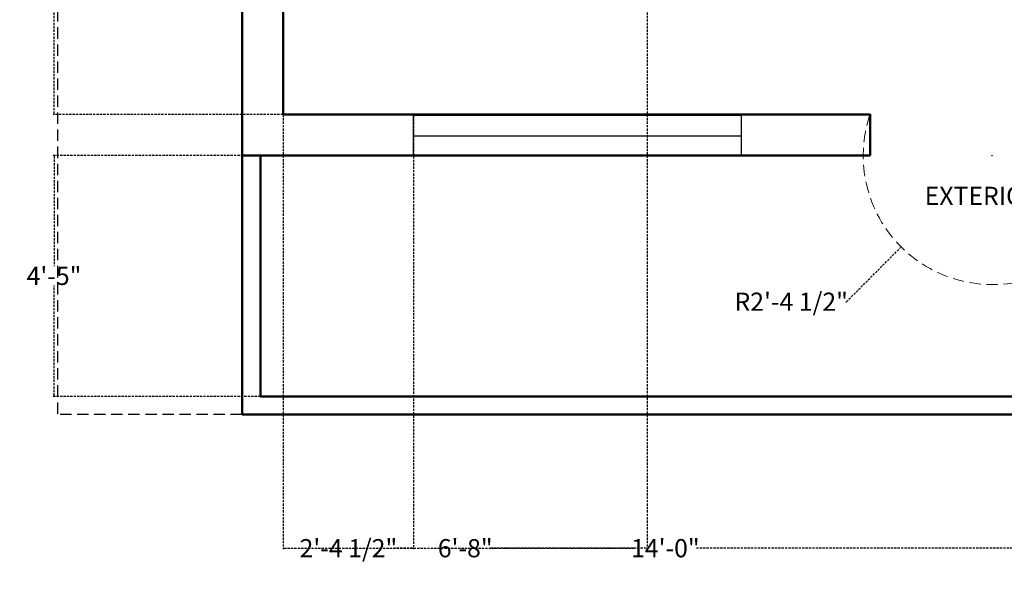
# Model space of a CAD drawing. Units: inches. Extents: x 513 to 1142, y 396 to 927.
# Tile 1 of 31: x 526 to 743, y 396 to 518. Entities that reach past the tile are written whole.
import ezdxf

# ---------------------------------------------------------------- set-up
doc = ezdxf.new("R2010")
doc.units = ezdxf.units.IN
doc.header["$MEASUREMENT"] = 0
doc.linetypes.add('DASHED', pattern=[0.75, 0.5, -0.25])
for name, color, linetype, lineweight in [('A-ANNO-DIMS', 2, 'DASHED', 18), ('A-DOOR-SWNG', 4, 'DASHED', 13), ('A-WALL', 7, 'Continuous', 50), ('windows', 172, 'Continuous', 25)]:
    doc.layers.add(name, color=color, linetype=linetype, lineweight=lineweight)
doc.styles.get("Standard").update_dxf_attribs({"font": 'arial.ttf'})
doc.dimstyles.get("Standard").update_dxf_attribs({"dimtxt": 4, "dimasz": 0.18, "dimexe": 0.18, "dimexo": 0.0625, "dimgap": 0.09, "dimtad": 0, "dimtih": 1, "dimtoh": 1, "dimdec": 0, "dimrnd": 6, "dimzin": 0, "dimdsep": 46, "dimlunit": 3, "dimtxsty": 'Standard', "dimcen": 0.09, "dimadec": 0, "dimazin": 0, "dimtfac": 1, "dimtdec": 0, "dimtofl": 0, "dimtmove": 0, "dimatfit": 3, "dimfxl": 1, "dimtolj": 1, "dimtzin": 0, "dimarcsym": 0})

# ---------------------------------------------------------------- blocks, each defined once
blk = doc.blocks.new('*D104')
at = {"layer": 'A-ANNO-DIMS', "color": 0, "lineweight": -2, "ltscale": 5, "transparency": 16777216}
for p, q in [((574.93, 879.16), (534.25, 879.16)), ((534.43, 878.98), (534.43, 657.29)), ((534.43, 431.34), (534.43, 653.02)), ((574.93, 431.16), (534.25, 431.16))]:
    blk.add_line(p, q, dxfattribs=at)
at = {"layer": 'A-ANNO-DIMS', "color": 0, "ltscale": 5, "transparency": 16777216}
for points in [[(534.4, 878.98), (534.46, 878.98), (534.43, 879.16)], [(534.4, 431.34), (534.46, 431.34), (534.43, 431.16)]]:
    blk.add_solid(points, dxfattribs=at)
at = {"layer": 'Defpoints', "color": 0, "ltscale": 5, "transparency": 16777216}
for p in [(575, 879.16), (534.43, 431.16), (575, 431.16)]:
    blk.add_point(p, dxfattribs=at)
at = {"layer": 'A-ANNO-DIMS', "color": 0, "ltscale": 5, "transparency": 16777216, "insert": (534.43, 655.16), "char_height": 4, "attachment_point": 5}
blk.add_mtext('\\A1;37\'-6"', dxfattribs=at)
blk = doc.blocks.new('WIN-72IN')
blk.add_line((0, 4.45), (72, 4.45))
blk.add_lwpolyline([(72, 9), (72, 0), (0, 0), (0, 9)], close=True)
blk = doc.blocks.new('*D125')
at = {"layer": 'A-ANNO-DIMS', "color": 0, "lineweight": -2, "transparency": 16777216}
for p, q in [((752.06, 497.26), (757.58, 497.26)), ((757.4, 497.08), (757.4, 481.42)), ((757.4, 461.44), (757.4, 477.1)), ((752.06, 461.26), (757.58, 461.26))]:
    blk.add_line(p, q, dxfattribs=at)
at = {"layer": 'A-ANNO-DIMS', "color": 0, "transparency": 16777216}
for points in [[(757.37, 497.08), (757.43, 497.08), (757.4, 497.26)], [(757.37, 461.44), (757.43, 461.44), (757.4, 461.26)]]:
    blk.add_solid(points, dxfattribs=at)
at = {"layer": 'Defpoints', "color": 0, "transparency": 16777216}
for p in [(752, 497.26), (757.4, 497.26), (752, 461.26)]:
    blk.add_point(p, dxfattribs=at)
at = {"layer": 'A-ANNO-DIMS', "color": 0, "transparency": 16777216, "insert": (757.4, 479.26), "char_height": 4, "attachment_point": 5}
blk.add_mtext('\\A1;EXTERIOR LEAF 3\'-0" TYP.', dxfattribs=at)
blk = doc.blocks.new('*D142')
at = {"layer": 'A-ANNO-DIMS', "color": 0, "lineweight": -2, "transparency": 16777216}
for p, q in [((583.93, 637.16), (533.42, 637.16)), ((533.6, 636.98), (533.6, 569.29)), ((533.6, 497.34), (533.6, 565.03)), ((583.93, 497.16), (533.42, 497.16))]:
    blk.add_line(p, q, dxfattribs=at)
at = {"layer": 'A-ANNO-DIMS', "color": 0, "transparency": 16777216}
for points in [[(533.57, 636.98), (533.63, 636.98), (533.6, 637.16)], [(533.57, 497.34), (533.63, 497.34), (533.6, 497.16)]]:
    blk.add_solid(points, dxfattribs=at)
at = {"layer": 'Defpoints', "color": 0, "transparency": 16777216}
for p in [(533.6, 637.16), (584, 637.16), (584, 497.16)]:
    blk.add_point(p, dxfattribs=at)
at = {"layer": 'A-ANNO-DIMS', "color": 0, "transparency": 16777216, "insert": (533.6, 567.16), "char_height": 4, "attachment_point": 5}
blk.add_mtext('\\A1;11\'-8"', dxfattribs=at)
blk = doc.blocks.new('*D143')
at = {"layer": 'A-ANNO-DIMS', "color": 0, "lineweight": -2, "transparency": 16777216}
for p, q in [((578.93, 488.16), (533.42, 488.16)), ((533.6, 487.98), (533.6, 463.78)), ((533.6, 435.34), (533.6, 459.53)), ((578.93, 435.16), (533.42, 435.16))]:
    blk.add_line(p, q, dxfattribs=at)
at = {"layer": 'A-ANNO-DIMS', "color": 0, "transparency": 16777216}
for points in [[(533.57, 487.98), (533.63, 487.98), (533.6, 488.16)], [(533.57, 435.34), (533.63, 435.34), (533.6, 435.16)]]:
    blk.add_solid(points, dxfattribs=at)
at = {"layer": 'Defpoints', "color": 0, "transparency": 16777216}
for p in [(533.6, 488.16), (579, 488.16), (579, 435.16)]:
    blk.add_point(p, dxfattribs=at)
at = {"layer": 'A-ANNO-DIMS', "color": 0, "transparency": 16777216, "insert": (533.6, 461.66), "char_height": 4, "attachment_point": 5}
blk.add_mtext('\\A1;4\'-5"', dxfattribs=at)
blk = doc.blocks.new('*D144')
at = {"layer": 'A-ANNO-DIMS', "color": 0, "lineweight": -2, "transparency": 16777216}
for p, q in [((584, 497.1), (584, 401.58)), ((752, 497.1), (752, 401.58)), ((584.18, 401.76), (661.22, 401.76)), ((751.82, 401.76), (674.77, 401.76))]:
    blk.add_line(p, q, dxfattribs=at)
at = {"layer": 'A-ANNO-DIMS', "color": 0, "transparency": 16777216}
for points in [[(584.18, 401.79), (584.18, 401.73), (584, 401.76)], [(751.82, 401.79), (751.82, 401.73), (752, 401.76)]]:
    blk.add_solid(points, dxfattribs=at)
at = {"layer": 'Defpoints', "color": 0, "transparency": 16777216}
for p in [(584, 497.16), (752, 497.16), (752, 401.76)]:
    blk.add_point(p, dxfattribs=at)
at = {"layer": 'A-ANNO-DIMS', "color": 0, "transparency": 16777216, "insert": (668, 401.76), "char_height": 4, "attachment_point": 5}
blk.add_mtext('\\A1;14\'-0"', dxfattribs=at)
blk = doc.blocks.new('*D147')
at = {"layer": 'A-ANNO-DIMS', "color": 0, "lineweight": -2, "transparency": 16777216}
for p, q in [((584, 671.1), (584, 401.58)), ((664, 671.1), (664, 401.58)), ((584.18, 401.76), (618.58, 401.76)), ((663.82, 401.76), (629.41, 401.76))]:
    blk.add_line(p, q, dxfattribs=at)
at = {"layer": 'A-ANNO-DIMS', "color": 0, "transparency": 16777216}
for points in [[(584.18, 401.79), (584.18, 401.73), (584, 401.76)], [(663.82, 401.79), (663.82, 401.73), (664, 401.76)]]:
    blk.add_solid(points, dxfattribs=at)
at = {"layer": 'Defpoints', "color": 0, "transparency": 16777216}
for p in [(584, 671.16), (664, 671.16), (664, 401.76)]:
    blk.add_point(p, dxfattribs=at)
at = {"layer": 'A-ANNO-DIMS', "color": 0, "transparency": 16777216, "insert": (624, 401.76), "char_height": 4, "attachment_point": 5}
blk.add_mtext('\\A1;6\'-8"', dxfattribs=at)
blk = doc.blocks.new('*D156')
at = {"layer": 'A-ANNO-DIMS', "color": 0, "lineweight": -2, "transparency": 16777216}
for p, q in [((584, 497.1), (584, 401.58)), ((612.64, 496.95), (612.64, 401.58)), ((584.18, 401.76), (588.21, 401.76)), ((612.46, 401.76), (608.42, 401.76))]:
    blk.add_line(p, q, dxfattribs=at)
at = {"layer": 'A-ANNO-DIMS', "color": 0, "transparency": 16777216}
for points in [[(584.18, 401.79), (584.18, 401.73), (584, 401.76)], [(612.46, 401.79), (612.46, 401.73), (612.64, 401.76)]]:
    blk.add_solid(points, dxfattribs=at)
at = {"layer": 'Defpoints', "color": 0, "transparency": 16777216}
for p in [(584, 497.16), (612.64, 497.01), (612.64, 401.76)]:
    blk.add_point(p, dxfattribs=at)
at = {"layer": 'A-ANNO-DIMS', "color": 0, "transparency": 16777216, "insert": (598.32, 401.76), "char_height": 4, "attachment_point": 5}
blk.add_mtext('\\A1;2\'-4 1/2"', dxfattribs=at)
blk = doc.blocks.new('*D178')
at = {"layer": 'A-ANNO-DIMS', "color": 0, "lineweight": -2, "transparency": 16777216}
for p, q in [((739.78, 488.11), (739.96, 488.11)), ((739.87, 488.02), (739.87, 488.2)), ((707.83, 455.98), (719.72, 467.9)), ((707.65, 455.98), (707.83, 455.98))]:
    blk.add_line(p, q, dxfattribs=at)
at = {"layer": 'A-ANNO-DIMS', "color": 0, "transparency": 16777216}
blk.add_solid([(719.7, 467.92), (719.74, 467.88), (719.85, 468.03)], dxfattribs=at)
at = {"layer": 'Defpoints', "color": 0, "transparency": 16777216}
for p in [(739.87, 488.11), (719.85, 468.03)]:
    blk.add_point(p, dxfattribs=at)
at = {"layer": 'A-ANNO-DIMS', "color": 0, "transparency": 16777216, "insert": (695.67, 455.98), "char_height": 4, "attachment_point": 5}
blk.add_mtext('\\A1;R2\'-4 1/2"', dxfattribs=at)

msp = doc.modelspace()

# ---------------------------------------------------------------- linework, layer by layer
at = {"layer": 'A-DOOR-SWNG', "ltscale": 5}
msp.add_arc((739.87, 488.11), 28.36, 161.3835, 288.7781, dxfattribs=at)
at = {"layer": 'A-WALL'}
for p, q in [((575, 879.16), (575, 431.16)), ((584, 637.16), (584, 497.16)), ((584, 497.16), (713, 497.16)), ((713, 488.16), (713, 497.26)), ((575, 488.16), (713, 488.16)), ((579, 488.16), (579, 435.16)), ((579, 435.16), (752, 435.16)), ((575, 431.16), (756, 431.16))]:
    msp.add_line(p, q, dxfattribs=at)

# ---------------------------------------------------------------- block references
at = {"layer": 'windows'}
msp.add_blockref('WIN-72IN', (612.64, 488.01), dxfattribs=at)

# ---------------------------------------------------------------- dimensions: what is measured, and where the dimension line sits
at = {"layer": 'A-ANNO-DIMS', "ltscale": 5}
dim = msp.add_linear_dim(base=(534.43, 431.16), p1=(575, 879.16), p2=(575, 431.16), angle=90, dimstyle='Standard', override={"dimclrd": 0, "dimclre": 0, "dimclrt": 0}, dxfattribs=at)
dim.commit()
dim.dimension.update_dxf_attribs({"geometry": '*D104', "text_midpoint": (534.43, 655.16)})
at = {"layer": 'A-ANNO-DIMS'}
for base, p1, p2, picture, middle in [((664, 401.76), (584, 671.16), (664, 671.16), '*D147', (624, 401.76)), ((752, 401.76), (584, 497.16), (752, 497.16), '*D144', (668, 401.76)), ((612.64, 401.76), (584, 497.16), (612.64, 497.01), '*D156', (598.32, 401.76))]:
    dim = msp.add_linear_dim(base=base, p1=p1, p2=p2, dimstyle='Standard', override={"dimdec": 1, "dimlfac": 1, "dimrnd": 0, "dimzin": 1, "dimdsep": 46, "dimlunit": 4, "dimfrac": 2}, dxfattribs=at)
    dim.commit()
    dim.dimension.update_dxf_attribs({"geometry": picture, "text_midpoint": middle})
for base, p1, p2, picture, middle in [((533.6, 637.16), (584, 497.16), (584, 637.16), '*D142', (533.6, 567.16)), ((533.6, 488.16), (579, 435.16), (579, 488.16), '*D143', (533.6, 461.66))]:
    dim = msp.add_linear_dim(base=base, p1=p1, p2=p2, angle=90, dimstyle='Standard', override={"dimdec": 1, "dimlfac": 1, "dimrnd": 0, "dimzin": 1, "dimdsep": 46, "dimlunit": 4, "dimfrac": 2}, dxfattribs=at)
    dim.commit()
    dim.dimension.update_dxf_attribs({"geometry": picture, "text_midpoint": middle})
dim = msp.add_linear_dim(base=(757.4, 497.26), p1=(752, 461.26), p2=(752, 497.26), angle=90, text='EXTERIOR LEAF <> TYP.', dimstyle='Standard', override={"dimdec": 1, "dimlfac": 1, "dimrnd": 0, "dimzin": 1, "dimdsep": 46, "dimlunit": 4, "dimfrac": 2}, dxfattribs=at)
dim.commit()
dim.dimension.update_dxf_attribs({"geometry": '*D125', "text_midpoint": (757.4, 479.26)})
dim = msp.add_radius_dim(center=(739.87, 488.11), mpoint=(719.85, 468.03), dimstyle='Standard', override={"dimdec": 1, "dimlfac": 1, "dimrnd": 0, "dimzin": 1, "dimdsep": 46, "dimlunit": 4, "dimfrac": 2}, dxfattribs=at)
dim.commit()
dim.dimension.update_dxf_attribs({"geometry": '*D178', "text_midpoint": (695.67, 455.98), "dimtype": 164})

doc.saveas('drawing.dxf')
